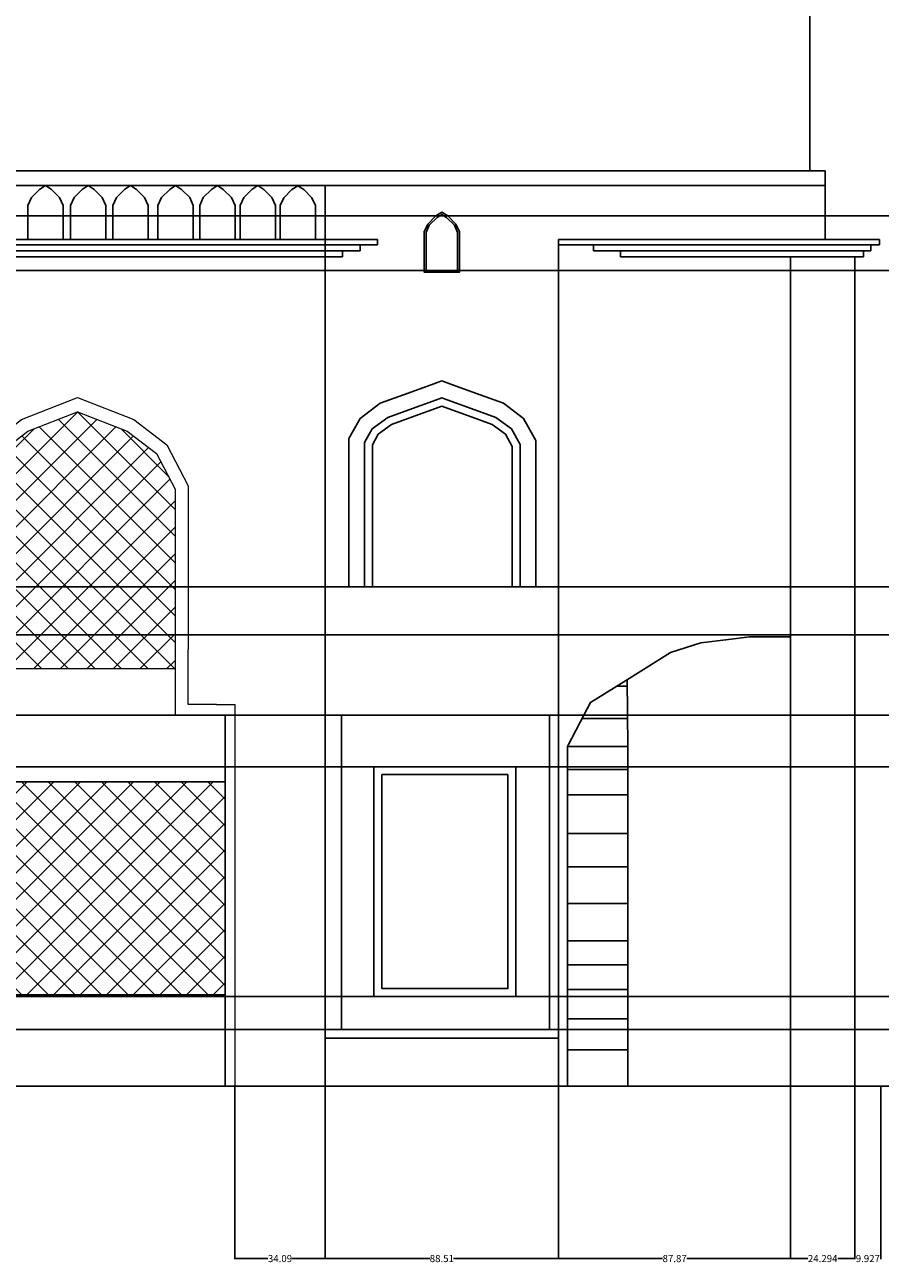
# Model space of a CAD drawing. Units: inches. Extents: x 2 to 1442, y 20 to 729.
# Tile 6 of 8: x 897 to 1221, y 20 to 489. Entities that reach past the tile are written whole.
import ezdxf

# ---------------------------------------------------------------- set-up
doc = ezdxf.new("R2010")
doc.units = ezdxf.units.IN
doc.header["$MEASUREMENT"] = 0
for name, color, linetype, lineweight in [('A-ANNO-DIMS', 2, 'Continuous', 18), ('A-ELEV', 7, 'Continuous', 25), ('A-GLAZ', 4, 'Continuous', 18), ('A-GLAZ-PATT', 9, 'Continuous', 13)]:
    doc.layers.add(name, color=color, linetype=linetype, lineweight=lineweight)
doc.styles.get("Standard").update_dxf_attribs({"font": 'arial.ttf'})
doc.dimstyles.get("Standard").update_dxf_attribs({"dimtxt": 2.6875, "dimasz": 0.18, "dimexe": 0.18, "dimexo": 0.0625, "dimgap": 0.09, "dimtad": 0, "dimtih": 1, "dimtoh": 1, "dimdec": 4, "dimzin": 0, "dimdsep": 46, "dimlunit": 4, "dimtxsty": 'Standard', "dimcen": 0.09, "dimadec": 0, "dimazin": 0, "dimtfac": 1, "dimtdec": 4, "dimtofl": 0, "dimtmove": 0, "dimatfit": 3, "dimfxl": 1, "dimtolj": 1, "dimtzin": 0, "dimarcsym": 0})

# ---------------------------------------------------------------- blocks, each defined once
blk = doc.blocks.new('WIN-JALI-PANEL')
for p, q in [((17.71, 144.52), (17.71, 165.38)), ((22.71, 165.38), (22.71, 158.15)), ((95.66, 165.25), (95.66, 158.15)), ((100.66, 165.25), (100.66, 143.52)), ((95.66, 158.15), (22.71, 158.15)), ((22.71, 158.15), (22.71, 140.52)), ((95.66, 158.15), (95.66, 140.52)), ((0, 0), (0, 144.52)), ((7.01, 144.52), (0, 144.52)), ((7.01, 144.52), (17.71, 144.52)), ((107.81, 143.52), (100.66, 143.52)), ((107.81, 143.52), (118.87, 143.52)), ((118.87, 143.52), (118.87, 100.88)), ((118.87, 100.88), (118.87, 0))]:
    blk.add_line(p, q)
for points in [[(100.66, 165.25), (100.66, 224.45), (100.65, 229.2), (93.44, 242.86), (80.93, 252.42), (59.66, 260.79), (38.39, 252.42), (25.88, 242.86), (17.71, 227.39), (17.71, 165.38)], [(95.66, 165.25), (95.66, 224.45), (95.66, 227.96), (89.53, 239.55), (78.45, 248.02), (59.66, 255.41), (40.87, 248.02), (29.79, 239.55), (22.71, 226.15), (22.71, 165.38)]]:
    blk.add_lwpolyline(points)
blk = doc.blocks.new('*D24')
at = {"layer": 'A-ANNO-DIMS', "color": 0, "lineweight": -2, "transparency": 16777216}
for p, q in [((976.59, 87.21), (976.59, 21.84)), ((1010.69, 87.21), (1010.69, 21.84)), ((976.77, 22.02), (989.01, 22.02)), ((1010.51, 22.02), (998.27, 22.02))]:
    blk.add_line(p, q, dxfattribs=at)
at = {"layer": 'A-ANNO-DIMS', "color": 0, "transparency": 16777216}
for points in [[(976.77, 22.05), (976.77, 21.99), (976.59, 22.02)], [(1010.51, 22.05), (1010.51, 21.99), (1010.69, 22.02)]]:
    blk.add_solid(points, dxfattribs=at)
at = {"layer": 'Defpoints', "color": 0, "transparency": 16777216}
for p in [(976.59, 87.27), (1010.69, 87.27), (1010.69, 22.02)]:
    blk.add_point(p, dxfattribs=at)
at = {"layer": 'A-ANNO-DIMS', "color": 0, "transparency": 16777216, "insert": (993.64, 22.02), "char_height": 2.688, "attachment_point": 5}
blk.add_mtext('\\A1;34.09', dxfattribs=at)
blk = doc.blocks.new('*D25')
at = {"layer": 'A-ANNO-DIMS', "color": 0, "lineweight": -2, "transparency": 16777216}
for p, q in [((1010.69, 87.21), (1010.69, 21.84)), ((1099.2, 87.21), (1099.2, 21.84)), ((1010.87, 22.02), (1050.58, 22.02)), ((1099.02, 22.02), (1059.31, 22.02))]:
    blk.add_line(p, q, dxfattribs=at)
at = {"layer": 'A-ANNO-DIMS', "color": 0, "transparency": 16777216}
for points in [[(1010.87, 22.05), (1010.87, 21.99), (1010.69, 22.02)], [(1099.02, 22.05), (1099.02, 21.99), (1099.2, 22.02)]]:
    blk.add_solid(points, dxfattribs=at)
at = {"layer": 'Defpoints', "color": 0, "transparency": 16777216}
for p in [(1010.69, 87.27), (1099.2, 87.27), (1099.2, 22.02)]:
    blk.add_point(p, dxfattribs=at)
at = {"layer": 'A-ANNO-DIMS', "color": 0, "transparency": 16777216, "insert": (1054.94, 22.02), "char_height": 2.688, "attachment_point": 5}
blk.add_mtext('\\A1;88.51', dxfattribs=at)
blk = doc.blocks.new('*D26')
at = {"layer": 'A-ANNO-DIMS', "color": 0, "lineweight": -2, "transparency": 16777216}
for p, q in [((1099.2, 87.21), (1099.2, 21.84)), ((1187.07, 87.21), (1187.07, 21.84)), ((1099.38, 22.02), (1138.51, 22.02)), ((1186.89, 22.02), (1147.76, 22.02))]:
    blk.add_line(p, q, dxfattribs=at)
at = {"layer": 'A-ANNO-DIMS', "color": 0, "transparency": 16777216}
for points in [[(1099.38, 22.05), (1099.38, 21.99), (1099.2, 22.02)], [(1186.89, 22.05), (1186.89, 21.99), (1187.07, 22.02)]]:
    blk.add_solid(points, dxfattribs=at)
at = {"layer": 'Defpoints', "color": 0, "transparency": 16777216}
for p in [(1099.2, 87.27), (1187.07, 87.27), (1187.07, 22.02)]:
    blk.add_point(p, dxfattribs=at)
at = {"layer": 'A-ANNO-DIMS', "color": 0, "transparency": 16777216, "insert": (1143.14, 22.02), "char_height": 2.688, "attachment_point": 5}
blk.add_mtext('\\A1;87.87', dxfattribs=at)
blk = doc.blocks.new('*D27')
at = {"layer": 'A-ANNO-DIMS', "color": 0, "lineweight": -2, "transparency": 16777216}
for p, q in [((1187.07, 87.21), (1187.07, 21.84)), ((1211.37, 87.21), (1211.37, 21.84)), ((1187.25, 22.02), (1193.54, 22.02)), ((1211.19, 22.02), (1204.91, 22.02))]:
    blk.add_line(p, q, dxfattribs=at)
at = {"layer": 'A-ANNO-DIMS', "color": 0, "transparency": 16777216}
for points in [[(1187.25, 22.05), (1187.25, 21.99), (1187.07, 22.02)], [(1211.19, 22.05), (1211.19, 21.99), (1211.37, 22.02)]]:
    blk.add_solid(points, dxfattribs=at)
at = {"layer": 'Defpoints', "color": 0, "transparency": 16777216}
for p in [(1187.07, 87.27), (1211.37, 87.27), (1211.37, 22.02)]:
    blk.add_point(p, dxfattribs=at)
at = {"layer": 'A-ANNO-DIMS', "color": 0, "transparency": 16777216, "insert": (1199.22, 22.02), "char_height": 2.688, "attachment_point": 5}
blk.add_mtext('\\A1;24.294', dxfattribs=at)
blk = doc.blocks.new('*D28')
at = {"layer": 'A-ANNO-DIMS', "color": 0, "lineweight": -2, "transparency": 16777216}
for p, q in [((1211.37, 87.21), (1211.37, 21.84)), ((1221.3, 87.21), (1221.3, 21.84)), ((1211.55, 22.02), (1211.71, 22.02)), ((1221.12, 22.02), (1220.96, 22.02))]:
    blk.add_line(p, q, dxfattribs=at)
at = {"layer": 'A-ANNO-DIMS', "color": 0, "transparency": 16777216}
for points in [[(1211.55, 22.05), (1211.55, 21.99), (1211.37, 22.02)], [(1221.12, 22.05), (1221.12, 21.99), (1221.3, 22.02)]]:
    blk.add_solid(points, dxfattribs=at)
at = {"layer": 'Defpoints', "color": 0, "transparency": 16777216}
for p in [(1211.37, 87.27), (1221.3, 87.27), (1221.3, 22.02)]:
    blk.add_point(p, dxfattribs=at)
at = {"layer": 'A-ANNO-DIMS', "color": 0, "transparency": 16777216, "insert": (1216.33, 22.02), "char_height": 2.688, "attachment_point": 5}
blk.add_mtext('\\A1;9.927', dxfattribs=at)
blk = doc.blocks.new('*D33')
at = {"layer": 'A-ANNO-DIMS', "color": 0, "lineweight": -2, "transparency": 16777216}
for p, q in [((722.06, 661.5), (1436.55, 661.5)), ((1436.37, 661.32), (1436.37, 375.85)), ((1436.37, 87.45), (1436.37, 372.92)), ((1371.19, 87.27), (1436.55, 87.27))]:
    blk.add_line(p, q, dxfattribs=at)
at = {"layer": 'A-ANNO-DIMS', "color": 0, "transparency": 16777216}
for points in [[(1436.34, 661.32), (1436.4, 661.32), (1436.37, 661.5)], [(1436.34, 87.45), (1436.4, 87.45), (1436.37, 87.27)]]:
    blk.add_solid(points, dxfattribs=at)
at = {"layer": 'Defpoints', "color": 0, "transparency": 16777216}
for p in [(722, 661.5), (1436.37, 661.5), (1371.12, 87.27)]:
    blk.add_point(p, dxfattribs=at)
at = {"layer": 'A-ANNO-DIMS', "color": 0, "transparency": 16777216, "insert": (1436.37, 374.39), "char_height": 2.688, "attachment_point": 5}
blk.add_mtext('\\A1;574.2', dxfattribs=at)
blk = doc.blocks.new('*D50')
at = {"layer": 'A-ANNO-DIMS', "color": 0, "lineweight": -2, "transparency": 16777216}
for p, q in [((433.03, 108.8), (1436.55, 108.8)), ((1436.37, 108.62), (1436.37, 99.5)), ((1436.37, 87.45), (1436.37, 96.57)), ((433.03, 87.27), (1436.55, 87.27))]:
    blk.add_line(p, q, dxfattribs=at)
at = {"layer": 'A-ANNO-DIMS', "color": 0, "transparency": 16777216}
for points in [[(1436.34, 108.62), (1436.4, 108.62), (1436.37, 108.8)], [(1436.34, 87.45), (1436.4, 87.45), (1436.37, 87.27)]]:
    blk.add_solid(points, dxfattribs=at)
at = {"layer": 'Defpoints', "color": 0, "transparency": 16777216}
for p in [(432.97, 108.8), (1436.37, 108.8), (432.97, 87.27)]:
    blk.add_point(p, dxfattribs=at)
at = {"layer": 'A-ANNO-DIMS', "color": 0, "transparency": 16777216, "insert": (1436.37, 98.04), "char_height": 2.688, "attachment_point": 5}
blk.add_mtext('\\A1;21.53', dxfattribs=at)
blk = doc.blocks.new('*D51')
at = {"layer": 'A-ANNO-DIMS', "color": 0, "lineweight": -2, "transparency": 16777216}
for p, q in [((426.83, 227.79), (1436.55, 227.79)), ((1436.37, 227.61), (1436.37, 169.76)), ((1436.37, 108.98), (1436.37, 166.83)), ((433.03, 108.8), (1436.55, 108.8))]:
    blk.add_line(p, q, dxfattribs=at)
at = {"layer": 'A-ANNO-DIMS', "color": 0, "transparency": 16777216}
for points in [[(1436.34, 227.61), (1436.4, 227.61), (1436.37, 227.79)], [(1436.34, 108.98), (1436.4, 108.98), (1436.37, 108.8)]]:
    blk.add_solid(points, dxfattribs=at)
at = {"layer": 'Defpoints', "color": 0, "transparency": 16777216}
for p in [(426.77, 227.79), (1436.37, 227.79), (432.97, 108.8)]:
    blk.add_point(p, dxfattribs=at)
at = {"layer": 'A-ANNO-DIMS', "color": 0, "transparency": 16777216, "insert": (1436.37, 168.3), "char_height": 2.688, "attachment_point": 5}
blk.add_mtext('\\A1;118.99', dxfattribs=at)
blk = doc.blocks.new('*D52')
at = {"layer": 'A-ANNO-DIMS', "color": 0, "lineweight": -2, "transparency": 16777216}
for p, q in [((433.03, 258.25), (1436.55, 258.25)), ((1436.37, 258.07), (1436.37, 244.49)), ((1436.37, 227.97), (1436.37, 241.56)), ((426.83, 227.79), (1436.55, 227.79))]:
    blk.add_line(p, q, dxfattribs=at)
at = {"layer": 'A-ANNO-DIMS', "color": 0, "transparency": 16777216}
for points in [[(1436.34, 258.07), (1436.4, 258.07), (1436.37, 258.25)], [(1436.34, 227.97), (1436.4, 227.97), (1436.37, 227.79)]]:
    blk.add_solid(points, dxfattribs=at)
at = {"layer": 'Defpoints', "color": 0, "transparency": 16777216}
for p in [(432.97, 258.25), (1436.37, 258.25), (426.77, 227.79)]:
    blk.add_point(p, dxfattribs=at)
at = {"layer": 'A-ANNO-DIMS', "color": 0, "transparency": 16777216, "insert": (1436.37, 243.02), "char_height": 2.688, "attachment_point": 5}
blk.add_mtext('\\A1;30.464', dxfattribs=at)
blk = doc.blocks.new('*D53')
at = {"layer": 'A-ANNO-DIMS', "color": 0, "lineweight": -2, "transparency": 16777216}
for p, q in [((433.03, 276.44), (1436.55, 276.44)), ((1436.37, 276.26), (1436.37, 268.81)), ((1436.37, 258.43), (1436.37, 265.89)), ((433.03, 258.25), (1436.55, 258.25))]:
    blk.add_line(p, q, dxfattribs=at)
at = {"layer": 'A-ANNO-DIMS', "color": 0, "transparency": 16777216}
for points in [[(1436.34, 276.26), (1436.4, 276.26), (1436.37, 276.44)], [(1436.34, 258.43), (1436.4, 258.43), (1436.37, 258.25)]]:
    blk.add_solid(points, dxfattribs=at)
at = {"layer": 'Defpoints', "color": 0, "transparency": 16777216}
for p in [(432.97, 276.44), (1436.37, 276.44), (432.97, 258.25)]:
    blk.add_point(p, dxfattribs=at)
at = {"layer": 'A-ANNO-DIMS', "color": 0, "transparency": 16777216, "insert": (1436.37, 267.35), "char_height": 2.688, "attachment_point": 5}
blk.add_mtext('\\A1;18.19', dxfattribs=at)
blk = doc.blocks.new('*D55')
at = {"layer": 'A-ANNO-DIMS', "color": 0, "lineweight": -2, "transparency": 16777216}
for p, q in [((391.01, 416.82), (1436.55, 416.82)), ((1436.37, 416.64), (1436.37, 407.98)), ((1436.37, 396.4), (1436.37, 405.06)), ((394.77, 396.22), (1436.55, 396.22))]:
    blk.add_line(p, q, dxfattribs=at)
at = {"layer": 'A-ANNO-DIMS', "color": 0, "transparency": 16777216}
for points in [[(1436.34, 416.64), (1436.4, 416.64), (1436.37, 416.82)], [(1436.34, 396.4), (1436.4, 396.4), (1436.37, 396.22)]]:
    blk.add_solid(points, dxfattribs=at)
at = {"layer": 'Defpoints', "color": 0, "transparency": 16777216}
for p in [(390.95, 416.82), (1436.37, 416.82), (394.7, 396.22)]:
    blk.add_point(p, dxfattribs=at)
at = {"layer": 'A-ANNO-DIMS', "color": 0, "transparency": 16777216, "insert": (1436.37, 406.52), "char_height": 2.688, "attachment_point": 5}
blk.add_mtext('\\A1;20.605', dxfattribs=at)
blk = doc.blocks.new('*D60')
at = {"layer": 'A-ANNO-DIMS', "color": 0, "lineweight": -2, "transparency": 16777216}
for p, q in [((414.48, 208.27), (1436.55, 208.27)), ((1436.37, 208.09), (1436.37, 166.24)), ((1436.37, 121.46), (1436.37, 163.32)), ((414.48, 121.28), (1436.55, 121.28))]:
    blk.add_line(p, q, dxfattribs=at)
at = {"layer": 'A-ANNO-DIMS', "color": 0, "transparency": 16777216}
for points in [[(1436.34, 208.09), (1436.4, 208.09), (1436.37, 208.27)], [(1436.34, 121.46), (1436.4, 121.46), (1436.37, 121.28)]]:
    blk.add_solid(points, dxfattribs=at)
at = {"layer": 'Defpoints', "color": 0, "transparency": 16777216}
for p in [(414.42, 208.27), (1436.37, 208.27), (414.42, 121.28)]:
    blk.add_point(p, dxfattribs=at)
at = {"layer": 'A-ANNO-DIMS', "color": 0, "transparency": 16777216, "insert": (1436.37, 164.78), "char_height": 2.688, "attachment_point": 5}
blk.add_mtext('\\A1;86.99', dxfattribs=at)

msp = doc.modelspace()

# ---------------------------------------------------------------- hatches: boundary and pattern name
at = {"layer": 'A-GLAZ-PATT'}
h = msp.add_hatch(dxfattribs=at)
h.set_pattern_fill('ANSI37', color=256, scale=57)
h.paths.add_polyline_path([(916.9314, 342.6839), (898.144, 335.2949), (887.0591, 326.8249), (880.9371, 315.2306), (880.9314, 311.7186), (880.9314, 252.5179), (880.9314, 245.4201), (953.8787, 245.4201), (953.8787, 252.6544), (953.8787, 313.4256), (946.8037, 326.8249), (935.7187, 335.2949)])
h.paths.add_polyline_path([(861.0256, 202.5842), (861.0256, 121.871), (972.8371, 121.871), (972.8371, 202.5842)])

# ---------------------------------------------------------------- linework, layer by layer
at = {"layer": 'A-ELEV'}
for p, q in [((1194.3036, 520.5823), (1194.3036, 471.2714)), ((1194.3036, 471.2714), (1194.3036, 433.9259)), ((1012.4347, 433.9259), (721.8257, 433.9259)), ((1038.5185, 433.9259), (1012.4347, 433.9259)), ((1194.3036, 433.9259), (1038.5185, 433.9259)), ((1194.3036, 433.9259), (1198.383, 433.9259)), ((1198.383, 433.9259), (1200.1922, 433.9259)), ((1200.1922, 433.9259), (1200.1922, 422.7015)), ((1010.6856, 428.3137), (726.6831, 428.3137)), ((1038.4061, 428.3137), (1010.6856, 428.3137)), ((1010.6856, 428.3137), (1010.6856, 87.2714)), ((1200.1922, 428.3137), (1038.4061, 428.3137)), ((1200.1922, 422.7015), (1200.1922, 407.8873)), ((1010.6856, 403.6578), (721.8257, 403.6578)), ((1010.6856, 407.8873), (725.555, 407.8873)), ((1010.6856, 405.9114), (728.2857, 405.9114)), ((1010.6856, 407.8873), (1030.593, 407.8873)), ((1030.593, 405.9114), (1010.6856, 405.9114)), ((1024.0109, 403.6578), (1010.6856, 403.6578)), ((1017.3482, 403.6578), (1017.3482, 401.3516)), ((1024.0109, 405.9114), (1024.0109, 403.6578)), ((1030.593, 407.8873), (1030.593, 405.9114)), ((1099.2001, 87.2714), (1099.2001, 407.8873)), ((1099.2001, 407.8873), (1139.2053, 407.8873)), ((1107.7684, 405.9114), (1099.2001, 405.9114)), ((1139.2053, 405.9114), (1107.7684, 405.9114)), ((1107.7684, 405.9114), (1107.7684, 405.9114)), ((1112.3438, 403.6578), (1112.3438, 405.9114)), ((1144.164, 403.6578), (1112.3438, 403.6578)), ((1122.6419, 401.3516), (1122.6419, 403.6578)), ((1152.0898, 407.8873), (1139.2053, 407.8873)), ((1139.2053, 405.9114), (1152.3627, 405.9114)), ((1194.3036, 403.6578), (1144.164, 403.6578)), ((1194.3036, 407.8873), (1152.0898, 407.8873)), ((1194.3036, 405.9114), (1152.3627, 405.9114)), ((1200.1922, 407.8873), (1194.3036, 407.8873)), ((1220.752, 405.9114), (1194.3036, 405.9114)), ((1217.4785, 403.6578), (1194.3036, 403.6578)), ((1200.1922, 407.8873), (1220.752, 407.8873)), ((1214.637, 403.6578), (1214.637, 401.3516)), ((1217.4785, 405.9114), (1217.4785, 403.6578)), ((1220.752, 407.8873), (1220.752, 405.9114)), ((1010.6856, 401.3516), (723.427, 401.3516)), ((1017.3482, 401.3516), (1010.6856, 401.3516)), ((1152.5553, 401.3516), (1122.6419, 401.3516)), ((1214.637, 401.3516), (1152.5553, 401.3516)), ((1187.0748, 401.3516), (1187.0748, 87.2714)), ((1211.369, 401.3516), (1211.369, 87.2714)), ((1099.2001, 276.443), (1010.6856, 276.443)), ((1099.2001, 258.2539), (1010.6856, 258.2539)), ((1125.404, 215.9163), (1125.2087, 241.3024)), ((1125.2279, 238.8156), (1121.1955, 238.7967)), ((1125.3229, 226.4671), (1108.0799, 226.4671)), ((1125.404, 215.9163), (1102.5891, 215.9163)), ((1125.404, 87.2714), (1125.404, 215.9163)), ((1125.404, 207.1602), (1102.5891, 207.1602)), ((972.8371, 202.5842), (861.0256, 202.5842)), ((1125.404, 197.6038), (1102.5891, 197.6038)), ((1125.404, 183.0302), (1102.5891, 183.0302)), ((1125.404, 170.3214), (1102.5891, 170.3214)), ((1125.404, 156.4645), (1102.5891, 156.4645)), ((1125.404, 142.3688), (1102.5891, 142.3688)), ((1125.404, 133.2901), (1102.5891, 133.2901)), ((1125.404, 123.9726), (1102.5891, 123.9726)), ((972.8371, 121.871), (861.0256, 121.871)), ((1125.404, 112.7437), (1102.5891, 112.7437)), ((1099.2001, 108.8033), (1010.6856, 108.8033)), ((1099.2001, 105.5085), (1010.6856, 105.5085)), ((1125.404, 101.0371), (1102.5891, 101.0371)), ((721.8257, 87.2714), (1371.1242, 87.2714))]:
    msp.add_line(p, q, dxfattribs=at)
for points in [[(898.1006, 420.8293), (899.4556, 423.7959), (902.5422, 426.88), (904.785, 428.3137), (907.0279, 426.88), (910.1145, 423.7959), (911.4695, 420.8293), (911.4695, 407.9694), (898.1006, 407.9694)], [(914.282, 420.8293), (915.637, 423.7959), (918.7235, 426.88), (920.9664, 428.3137), (923.2093, 426.88), (926.2959, 423.7959), (927.6509, 420.8293), (927.6509, 407.9694), (914.282, 407.9694)], [(930.299, 420.8293), (931.654, 423.7959), (934.7406, 426.88), (936.9835, 428.3137), (939.2263, 426.88), (942.3129, 423.7959), (943.6679, 420.8293), (943.6679, 407.9694), (930.299, 407.9694)], [(947.4124, 420.8293), (948.7674, 423.7959), (951.854, 426.88), (954.0969, 428.3137), (956.3397, 426.88), (959.4263, 423.7959), (960.7813, 420.8293), (960.7813, 407.9694), (947.4124, 407.9694)], [(963.2267, 420.8293), (964.5817, 423.7959), (967.6683, 426.88), (969.9111, 428.3137), (972.154, 426.88), (975.2406, 423.7959), (976.5956, 420.8293), (976.5956, 407.9694), (963.2267, 407.9694)], [(978.5679, 420.8293), (979.9229, 423.7959), (983.0095, 426.88), (985.2523, 428.3137), (987.4952, 426.88), (990.5818, 423.7959), (991.9368, 420.8293), (991.9368, 407.9694), (978.5679, 407.9694)], [(993.7113, 420.7472), (995.0664, 423.7138), (998.1529, 426.7979), (1000.3958, 428.2315), (1002.6387, 426.7979), (1005.7252, 423.7138), (1007.0803, 420.7472), (1007.0803, 407.8873), (993.7113, 407.8873)], [(1048.2584, 410.7704), (1049.6134, 413.737), (1052.7, 416.8211), (1054.9428, 418.2547), (1057.1857, 416.8211), (1060.2723, 413.737), (1061.6273, 410.7704), (1061.6273, 395.5258), (1048.2584, 395.5258)], [(1048.9485, 410.6202), (1050.1894, 413.3369), (1053.1348, 416.2799), (1054.9428, 417.4357), (1056.7509, 416.2799), (1059.6963, 413.3369), (1060.9372, 410.6202), (1060.9372, 396.2159), (1048.9485, 396.2159)], [(972.8371, 227.7901), (861.0256, 227.7901), (861.0256, 87.2714), (972.8371, 87.2714)], [(1095.669, 108.8033), (1016.8826, 108.8033), (1016.8826, 227.7901), (1095.669, 227.7901)], [(1082.9759, 208.2722), (1029.2296, 208.2722), (1029.2296, 121.2842), (1082.9759, 121.2842)], [(1079.9759, 205.2722), (1032.2296, 205.2722), (1032.2296, 124.2842), (1079.9759, 124.2842)]]:
    msp.add_lwpolyline(points, close=True, dxfattribs=at)
for points in [[(1019.7087, 276.443), (1019.7087, 332.5461), (1023.9462, 340.1919), (1031.5412, 345.8836), (1040.4287, 349.1128), (1050.8444, 352.8973), (1054.9428, 354.3865), (1059.0413, 352.8973), (1069.4569, 349.1128), (1078.3445, 345.8836), (1085.9394, 340.1919), (1090.5564, 331.8615), (1090.5564, 276.443)], [(1025.7087, 276.443), (1025.7087, 330.9946), (1028.5718, 336.1605), (1034.4269, 340.5483), (1042.4777, 343.4735), (1052.8934, 347.258), (1054.9428, 348.0027), (1056.9923, 347.258), (1067.4079, 343.4735), (1075.4588, 340.5483), (1081.3139, 336.1605), (1084.5564, 330.31), (1084.5564, 276.443)], [(1028.7087, 276.443), (1028.7087, 330.2188), (1030.8845, 334.1447), (1035.8698, 337.8807), (1043.5022, 340.6539), (1053.9179, 344.4384), (1054.9428, 344.8108), (1055.9678, 344.4384), (1066.3834, 340.6539), (1074.0159, 337.8807), (1079.0011, 334.1447), (1081.5564, 329.5342), (1081.5564, 276.443)], [(1141.5855, 251.5273), (1153.0294, 255.1671), (1163.5503, 256.4358), (1171.482, 257.3923), (1178.1527, 257.3923), (1187.0748, 257.3923)], [(1102.5891, 87.2714), (1102.5891, 215.9163), (1107.3729, 225.1085), (1111.272, 232.6009), (1122.8281, 239.816), (1132.2894, 245.7232), (1141.5855, 251.5273), (1141.5855, 251.5273)]]:
    msp.add_lwpolyline(points, dxfattribs=at)

# ---------------------------------------------------------------- block references
at = {"layer": 'A-GLAZ', "extrusion": (0, 0, -1), "zscale": -1}
msp.add_blockref('WIN-JALI-PANEL', (-976.5934, 87.271), dxfattribs=at)

# ---------------------------------------------------------------- dimensions: what is measured, and where the dimension line sits
at = {"layer": 'A-ANNO-DIMS'}
for base, p1, p2, override, picture, middle in [((1436.3742, 661.5), (1371.1242, 87.2714), (722, 661.5), {"dimdec": 1, "dimlfac": 1, "dimrnd": 0, "dimzin": 0, "dimdsep": 46, "dimlunit": 2}, '*D33', (1436.3742, 374.3857)), ((1436.3742, 416.8211), (394.7029, 396.2159), (390.9514, 416.8211), {"dimdec": 3, "dimlfac": 1, "dimrnd": 0, "dimzin": 0, "dimdsep": 46, "dimlunit": 2}, '*D55', (1436.3742, 406.5185)), ((1436.3742, 276.443), (432.9658, 258.2539), (432.9658, 276.443), {"dimdec": 2, "dimlfac": 1, "dimrnd": 0, "dimzin": 0, "dimdsep": 46, "dimlunit": 2}, '*D53', (1436.3742, 267.3485)), ((1436.3742, 258.2539), (426.7688, 227.7901), (432.9658, 258.2539), {"dimdec": 3, "dimlfac": 1, "dimrnd": 0, "dimzin": 0, "dimdsep": 46, "dimlunit": 2}, '*D52', (1436.3742, 243.022)), ((1436.3742, 227.7901), (432.9658, 108.8033), (426.7688, 227.7901), {"dimdec": 2, "dimlfac": 1, "dimrnd": 0, "dimzin": 0, "dimdsep": 46, "dimlunit": 2}, '*D51', (1436.3742, 168.2967)), ((1436.3742, 208.2722), (414.4218, 121.2842), (414.4218, 208.2722), {"dimdec": 2, "dimlfac": 1, "dimrnd": 0, "dimzin": 0, "dimdsep": 46, "dimlunit": 2}, '*D60', (1436.3742, 164.7782)), ((1436.3742, 108.8033), (432.9658, 87.2714), (432.9658, 108.8033), {"dimdec": 2, "dimlfac": 1, "dimrnd": 0, "dimzin": 0, "dimdsep": 46, "dimlunit": 2}, '*D50', (1436.3742, 98.0373))]:
    dim = msp.add_linear_dim(base=base, p1=p1, p2=p2, angle=90, dimstyle='Standard', override=override, dxfattribs=at)
    dim.commit()
    dim.dimension.update_dxf_attribs({"geometry": picture, "text_midpoint": middle})
for base, p1, p2, override, picture, middle in [((1010.6856, 22.0214), (976.5937, 87.2714), (1010.6856, 87.2714), {"dimdec": 2, "dimlfac": 1, "dimrnd": 0, "dimzin": 0, "dimdsep": 46, "dimlunit": 2}, '*D24', (993.6396, 22.0214)), ((1099.2001, 22.0214), (1010.6856, 87.2714), (1099.2001, 87.2714), {"dimdec": 2, "dimlfac": 1, "dimrnd": 0, "dimzin": 0, "dimdsep": 46, "dimlunit": 2}, '*D25', (1054.9428, 22.0214)), ((1187.0748, 22.0214), (1099.2001, 87.2714), (1187.0748, 87.2714), {"dimdec": 2, "dimlfac": 1, "dimrnd": 0, "dimzin": 0, "dimdsep": 46, "dimlunit": 2}, '*D26', (1143.1374, 22.0214)), ((1211.369, 22.0214), (1187.0748, 87.2714), (1211.369, 87.2714), {"dimdec": 3, "dimlfac": 1, "dimrnd": 0, "dimzin": 0, "dimdsep": 46, "dimlunit": 2}, '*D27', (1199.2219, 22.0214)), ((1221.296, 22.0214), (1211.369, 87.2714), (1221.296, 87.2714), {"dimdec": 3, "dimlfac": 1, "dimrnd": 0, "dimzin": 0, "dimdsep": 46, "dimlunit": 2}, '*D28', (1216.3325, 22.0214))]:
    dim = msp.add_linear_dim(base=base, p1=p1, p2=p2, dimstyle='Standard', override=override, dxfattribs=at)
    dim.commit()
    dim.dimension.update_dxf_attribs({"geometry": picture, "text_midpoint": middle})

doc.saveas('drawing.dxf')
